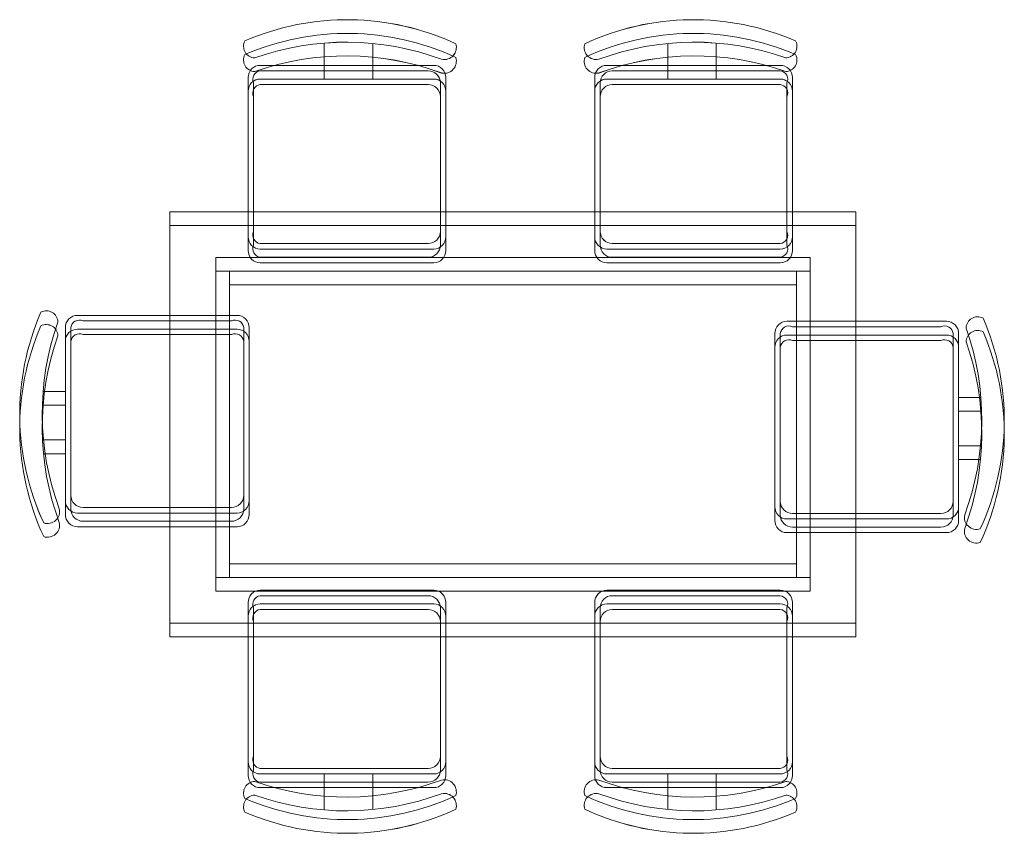
# Model space of a CAD drawing. Units: inches. Extents: x 963 to 2075, y 289 to 2657.
# Tile 90 of 98: x 1729 to 1781, y 2240 to 2282. Entities that reach past the tile are written whole.
import ezdxf

# ---------------------------------------------------------------- set-up
doc = ezdxf.new("R2010")
doc.units = ezdxf.units.IN
doc.layers.add('A-FURN', color=8, linetype='Continuous', lineweight=18)

msp = doc.modelspace()

# ---------------------------------------------------------------- linework, layer by layer
at = {"layer": 'A-FURN'}
for points in [[(1741.759, 2280.462, -0.175809), (1751.513, 2280.388, 0.578392), (1752.252, 2281.201, 0.214524), (1741.241, 2281.348, 0.552014), (1741.759, 2280.462, -0.065079)], [(1741.759, 2280.461, -0.175809), (1751.513, 2280.388, 0.578392), (1752.252, 2281.2, 0.214524), (1741.241, 2281.348, 0.552014), (1741.759, 2280.461, -0.065079)], [(1759.724, 2280.388, -0.578392), (1758.985, 2281.201, -0.214524), (1769.995, 2281.348, -0.552014), (1769.478, 2280.462, 0.175809), (1759.724, 2280.388)], [(1759.724, 2280.388, -0.578392), (1758.985, 2281.2, -0.214524), (1769.995, 2281.348, -0.552014), (1769.478, 2280.461, 0.175809), (1759.724, 2280.388)], [(1741.759, 2279.746, -0.175809), (1751.513, 2279.672, 0.578392), (1752.252, 2280.484, 0.214524), (1741.241, 2280.632, 0.552014), (1741.759, 2279.746, -0.065079)], [(1741.759, 2279.745, -0.175809), (1751.513, 2279.671, 0.578392), (1752.252, 2280.484, 0.214524), (1741.241, 2280.632, 0.552014), (1741.759, 2279.745, -0.065079)], [(1759.724, 2279.672, -0.578392), (1758.985, 2280.484, -0.214524), (1769.995, 2280.632, -0.552014), (1769.478, 2279.746, 0.175809), (1759.724, 2279.672)], [(1759.724, 2279.671, -0.578392), (1758.985, 2280.484, -0.214524), (1769.995, 2280.632, -0.552014), (1769.478, 2279.745, 0.175809), (1759.724, 2279.671)], [(1747.918, 2280.07), (1747.918, 2281.216, -0.064759)], [(1747.918, 2280.07), (1747.918, 2281.215, -0.064759)], [(1763.319, 2280.07), (1763.319, 2281.216, 0.064759)], [(1763.319, 2280.07), (1763.319, 2281.215, 0.064759)], [(1747.918, 2279.354), (1747.918, 2280.499, -0.064759)], [(1747.918, 2279.354), (1747.918, 2280.499, -0.064759)], [(1763.319, 2279.354), (1763.319, 2280.499, 0.064759)], [(1763.319, 2279.354), (1763.319, 2280.499, 0.064759)], [(1751.099, 2280.07), (1742.044, 2280.07, 0.414214), (1741.41, 2279.437), (1741.41, 2271.111, 0.414214), (1742.044, 2270.477), (1751.099, 2270.477, 0.414214), (1751.732, 2271.111), (1751.732, 2279.437, 0.414214), (1751.099, 2280.07)], [(1751.099, 2280.07), (1742.044, 2280.07, 0.414214), (1741.41, 2279.437), (1741.41, 2271.11, 0.414214), (1742.044, 2270.477), (1751.099, 2270.477, 0.414214), (1751.732, 2271.11), (1751.732, 2279.437, 0.414214), (1751.099, 2280.07)], [(1769.193, 2280.07, -0.414214), (1769.827, 2279.437), (1769.827, 2271.111, -0.414214), (1769.193, 2270.477), (1760.138, 2270.477, -0.414214), (1759.504, 2271.111), (1759.504, 2279.437, -0.414214), (1760.138, 2280.07), (1769.193, 2280.07)], [(1769.193, 2280.07, -0.414214), (1769.827, 2279.437), (1769.827, 2271.11, -0.414214), (1769.193, 2270.477), (1760.138, 2270.477, -0.414214), (1759.504, 2271.11), (1759.504, 2279.437, -0.414214), (1760.138, 2280.07), (1769.193, 2280.07)], [(1751.099, 2279.354), (1742.044, 2279.354, 0.414214), (1741.41, 2278.721), (1741.41, 2270.395, 0.414214), (1742.044, 2269.761), (1751.099, 2269.761, 0.414214), (1751.732, 2270.395), (1751.732, 2278.721, 0.414214), (1751.099, 2279.354)], [(1751.099, 2279.354), (1742.044, 2279.354, 0.414214), (1741.41, 2278.72), (1741.41, 2270.394, 0.414214), (1742.044, 2269.761), (1751.099, 2269.761, 0.414214), (1751.732, 2270.394), (1751.732, 2278.72, 0.414214), (1751.099, 2279.354)], [(1769.193, 2279.354, -0.414214), (1769.827, 2278.721), (1769.827, 2270.395, -0.414214), (1769.193, 2269.761), (1760.138, 2269.761, -0.414214), (1759.504, 2270.395), (1759.504, 2278.721, -0.414214), (1760.138, 2279.354), (1769.193, 2279.354)], [(1769.193, 2279.354, -0.414214), (1769.827, 2278.72), (1769.827, 2270.394, -0.414214), (1769.193, 2269.761), (1760.138, 2269.761, -0.414214), (1759.504, 2270.394), (1759.504, 2278.72, -0.414214), (1760.138, 2279.354), (1769.193, 2279.354)], [(1731.554, 2256.908, -0.578392), (1730.742, 2256.169, -0.214524), (1730.594, 2267.179, -0.552014), (1731.48, 2266.662, 0.175809), (1731.554, 2256.908)], [(1731.554, 2256.907, -0.578392), (1730.742, 2256.168, -0.214524), (1730.594, 2267.178, -0.552014), (1731.48, 2266.661, 0.175809), (1731.554, 2256.907)], [(1731.872, 2266.377, -0.414214), (1732.505, 2267.01), (1740.831, 2267.01, -0.414214), (1741.465, 2266.377), (1741.465, 2257.321, -0.414214), (1740.831, 2256.688), (1732.505, 2256.688, -0.414214), (1731.872, 2257.321), (1731.872, 2266.377)], [(1731.872, 2266.376, -0.414214), (1732.505, 2267.01), (1740.831, 2267.01, -0.414214), (1741.465, 2266.376), (1741.465, 2257.321, -0.414214), (1740.831, 2256.688), (1732.505, 2256.688, -0.414214), (1731.872, 2257.321), (1731.872, 2266.376)], [(1778.893, 2266.351, -0.175809), (1778.82, 2256.598, 0.578392), (1779.632, 2255.859, 0.214524), (1779.78, 2266.869, 0.552014), (1778.893, 2266.351, -0.065079)], [(1778.893, 2266.351, -0.175809), (1778.82, 2256.597, 0.578392), (1779.632, 2255.858, 0.214524), (1779.78, 2266.868, 0.552014), (1778.893, 2266.351, -0.065079)], [(1731.554, 2256.191, -0.578392), (1730.742, 2255.452, -0.214524), (1730.594, 2266.463, -0.552014), (1731.48, 2265.945, 0.175809), (1731.554, 2256.191)], [(1731.554, 2256.191, -0.578392), (1730.742, 2255.452, -0.214524), (1730.594, 2266.462, -0.552014), (1731.48, 2265.945, 0.175809), (1731.554, 2256.191)], [(1778.502, 2266.067, 0.414214), (1777.868, 2266.7), (1769.542, 2266.7, 0.414214), (1768.909, 2266.067), (1768.909, 2257.011, 0.414214), (1769.542, 2256.378), (1777.868, 2256.378, 0.414214), (1778.502, 2257.011), (1778.502, 2266.067)], [(1778.502, 2266.066, 0.414214), (1777.868, 2266.7), (1769.542, 2266.7, 0.414214), (1768.909, 2266.066), (1768.909, 2257.011, 0.414214), (1769.542, 2256.377), (1777.868, 2256.377, 0.414214), (1778.502, 2257.011), (1778.502, 2266.066)], [(1731.872, 2265.66, -0.414214), (1732.505, 2266.294), (1740.831, 2266.294, -0.414214), (1741.465, 2265.66), (1741.465, 2256.605, -0.414214), (1740.831, 2255.972), (1732.505, 2255.972, -0.414214), (1731.872, 2256.605), (1731.872, 2265.66)], [(1731.872, 2265.66, -0.414214), (1732.505, 2266.294), (1740.831, 2266.294, -0.414214), (1741.465, 2265.66), (1741.465, 2256.605, -0.414214), (1740.831, 2255.971), (1732.505, 2255.971, -0.414214), (1731.872, 2256.605), (1731.872, 2265.66)], [(1778.502, 2265.35, 0.414214), (1777.868, 2265.984), (1769.542, 2265.984, 0.414214), (1768.909, 2265.35), (1768.909, 2256.295, 0.414214), (1769.542, 2255.662), (1777.868, 2255.662, 0.414214), (1778.502, 2256.295), (1778.502, 2265.35)], [(1778.502, 2265.35, 0.414214), (1777.868, 2265.983), (1769.542, 2265.983, 0.414214), (1768.909, 2265.35), (1768.909, 2256.295, 0.414214), (1769.542, 2255.661), (1777.868, 2255.661, 0.414214), (1778.502, 2256.295), (1778.502, 2265.35)], [(1778.893, 2265.635, -0.175809), (1778.82, 2255.881, 0.578392), (1779.632, 2255.142, 0.214524), (1779.78, 2266.152, 0.552014), (1778.893, 2265.635, -0.065079)], [(1778.893, 2265.635, -0.175809), (1778.82, 2255.881, 0.578392), (1779.632, 2255.142, 0.214524), (1779.78, 2266.152, 0.552014), (1778.893, 2265.635, -0.065079)], [(1731.872, 2260.502), (1730.727, 2260.502, 0.064759)], [(1731.872, 2260.502), (1730.727, 2260.502, 0.064759)], [(1778.502, 2260.192), (1779.647, 2260.192, -0.064759)], [(1778.502, 2260.192), (1779.647, 2260.192, -0.064759)], [(1731.872, 2259.786), (1730.727, 2259.786, 0.064759)], [(1731.872, 2259.786), (1730.727, 2259.786, 0.064759)], [(1778.502, 2259.476), (1779.647, 2259.476, -0.064759)], [(1778.502, 2259.475), (1779.647, 2259.475, -0.064759)], [(1751.099, 2243.059), (1742.044, 2243.059, -0.414214), (1741.41, 2243.692), (1741.41, 2252.019, -0.414214), (1742.044, 2252.652), (1751.099, 2252.652, -0.414214), (1751.732, 2252.019), (1751.732, 2243.692, -0.414214), (1751.099, 2243.059)], [(1751.099, 2243.059), (1742.044, 2243.059, -0.414214), (1741.41, 2243.692), (1741.41, 2252.018, -0.414214), (1742.044, 2252.652), (1751.099, 2252.652, -0.414214), (1751.732, 2252.018), (1751.732, 2243.692, -0.414214), (1751.099, 2243.059)], [(1769.193, 2243.059, 0.414214), (1769.827, 2243.692), (1769.827, 2252.019, 0.414214), (1769.193, 2252.652), (1760.138, 2252.652, 0.414214), (1759.504, 2252.019), (1759.504, 2243.692, 0.414214), (1760.138, 2243.059), (1769.193, 2243.059)], [(1769.193, 2243.059, 0.414214), (1769.827, 2243.692), (1769.827, 2252.018, 0.414214), (1769.193, 2252.652), (1760.138, 2252.652, 0.414214), (1759.504, 2252.018), (1759.504, 2243.692, 0.414214), (1760.138, 2243.059), (1769.193, 2243.059)], [(1751.099, 2242.343), (1742.044, 2242.343, -0.414214), (1741.41, 2242.976), (1741.41, 2251.302, -0.414214), (1742.044, 2251.936), (1751.099, 2251.936, -0.414214), (1751.732, 2251.302), (1751.732, 2242.976, -0.414214), (1751.099, 2242.343)], [(1751.099, 2242.342), (1742.044, 2242.342, -0.414214), (1741.41, 2242.976), (1741.41, 2251.302, -0.414214), (1742.044, 2251.935), (1751.099, 2251.935, -0.414214), (1751.732, 2251.302), (1751.732, 2242.976, -0.414214), (1751.099, 2242.342)], [(1769.193, 2242.343, 0.414214), (1769.827, 2242.976), (1769.827, 2251.302, 0.414214), (1769.193, 2251.936), (1760.138, 2251.936, 0.414214), (1759.504, 2251.302), (1759.504, 2242.976, 0.414214), (1760.138, 2242.343), (1769.193, 2242.343)], [(1769.193, 2242.342, 0.414214), (1769.827, 2242.976), (1769.827, 2251.302, 0.414214), (1769.193, 2251.935), (1760.138, 2251.935, 0.414214), (1759.504, 2251.302), (1759.504, 2242.976, 0.414214), (1760.138, 2242.342), (1769.193, 2242.342)], [(1751.513, 2242.741, -0.578392), (1752.252, 2241.929, -0.214524), (1741.241, 2241.781, -0.552014), (1741.759, 2242.667, 0.175809), (1751.513, 2242.741)], [(1751.513, 2242.741, -0.578392), (1752.252, 2241.928, -0.214524), (1741.241, 2241.781, -0.552014), (1741.759, 2242.667, 0.175809), (1751.513, 2242.741)], [(1747.918, 2243.059), (1747.918, 2241.914, 0.064759)], [(1747.918, 2243.059), (1747.918, 2241.913, 0.064759)], [(1769.478, 2242.667, -0.175809), (1759.724, 2242.741, 0.578392), (1758.985, 2241.929, 0.214524), (1769.995, 2241.781, 0.552014), (1769.478, 2242.667, -0.065079)], [(1769.478, 2242.667, -0.175809), (1759.724, 2242.741, 0.578392), (1758.985, 2241.928, 0.214524), (1769.995, 2241.781, 0.552014), (1769.478, 2242.667, -0.065079)], [(1763.319, 2243.059), (1763.319, 2241.914, -0.064759)], [(1763.319, 2243.059), (1763.319, 2241.913, -0.064759)], [(1747.918, 2242.343), (1747.918, 2241.197, 0.064759)], [(1747.918, 2242.342), (1747.918, 2241.197, 0.064759)], [(1763.319, 2242.343), (1763.319, 2241.197, -0.064759)], [(1763.319, 2242.342), (1763.319, 2241.197, -0.064759)], [(1751.513, 2242.025, -0.578392), (1752.252, 2241.213, -0.214524), (1741.241, 2241.065, -0.552014), (1741.759, 2241.951, 0.175809), (1751.513, 2242.025)], [(1751.513, 2242.025, -0.578392), (1752.252, 2241.212, -0.214524), (1741.241, 2241.064, -0.552014), (1741.759, 2241.951, 0.175809), (1751.513, 2242.025)], [(1769.478, 2241.951, -0.175809), (1759.724, 2242.025, 0.578392), (1758.985, 2241.213, 0.214524), (1769.995, 2241.065, 0.552014), (1769.478, 2241.951, -0.065079)], [(1769.478, 2241.951, -0.175809), (1759.724, 2242.025, 0.578392), (1758.985, 2241.212, 0.214524), (1769.995, 2241.064, 0.552014), (1769.478, 2241.951, -0.065079)]]:
    msp.add_lwpolyline(points, format="xyb", dxfattribs=at)
for points in [[(1745.383, 2281.236), (1745.383, 2280.07)], [(1745.383, 2281.236), (1745.383, 2280.07)], [(1765.853, 2281.236), (1765.853, 2280.07)], [(1765.853, 2281.236), (1765.853, 2280.07)], [(1745.383, 2280.52), (1745.383, 2279.354)], [(1745.383, 2280.52), (1745.383, 2279.354)], [(1765.853, 2280.52), (1765.853, 2279.354)], [(1765.853, 2280.52), (1765.853, 2279.354)], [(1730.706, 2263.037), (1731.872, 2263.037)], [(1730.706, 2263.036), (1731.872, 2263.036)], [(1730.706, 2262.321), (1731.872, 2262.321)], [(1730.706, 2262.32), (1731.872, 2262.32)], [(1779.668, 2262.727), (1778.502, 2262.727)], [(1779.668, 2262.726), (1778.502, 2262.726)], [(1779.668, 2262.01), (1778.502, 2262.01)], [(1779.668, 2262.01), (1778.502, 2262.01)], [(1745.383, 2241.893), (1745.383, 2243.059)], [(1745.383, 2241.893), (1745.383, 2243.059)], [(1765.853, 2241.893), (1765.853, 2243.059)], [(1765.853, 2241.893), (1765.853, 2243.059)], [(1745.383, 2241.177), (1745.383, 2242.343)], [(1745.383, 2241.176), (1745.383, 2242.342)], [(1765.853, 2241.177), (1765.853, 2242.343)], [(1765.853, 2241.176), (1765.853, 2242.342)]]:
    msp.add_lwpolyline(points, dxfattribs=at)
for points in [[(1742.047, 2279.785), (1750.813, 2279.785, -0.414214), (1751.447, 2279.151), (1751.447, 2271.396, -0.414214), (1750.813, 2270.763), (1742.047, 2270.763, -0.512069), (1741.695, 2271.396), (1741.695, 2279.151, -0.512069)], [(1742.047, 2279.785), (1750.813, 2279.785, -0.414214), (1751.447, 2279.151), (1751.447, 2271.396, -0.414214), (1750.813, 2270.762), (1742.047, 2270.762, -0.512069), (1741.696, 2271.396), (1741.696, 2279.151, -0.512069)], [(1769.189, 2279.785), (1760.423, 2279.785, 0.414214), (1759.79, 2279.151), (1759.79, 2271.396, 0.414214), (1760.423, 2270.763), (1769.189, 2270.763, 0.512069), (1769.541, 2271.396), (1769.541, 2279.151, 0.512069)], [(1769.189, 2279.785), (1760.423, 2279.785, 0.414214), (1759.79, 2279.151), (1759.79, 2271.396, 0.414214), (1760.423, 2270.762), (1769.189, 2270.762, 0.512069), (1769.541, 2271.396), (1769.541, 2279.151, 0.512069)], [(1742.047, 2279.069), (1750.813, 2279.069, -0.414214), (1751.447, 2278.435), (1751.447, 2270.68, -0.414214), (1750.813, 2270.046), (1742.047, 2270.046, -0.512069), (1741.695, 2270.68), (1741.695, 2278.435, -0.512069)], [(1742.047, 2279.068), (1750.813, 2279.068, -0.414214), (1751.447, 2278.435), (1751.447, 2270.68, -0.414214), (1750.813, 2270.046), (1742.047, 2270.046, -0.512069), (1741.696, 2270.68), (1741.696, 2278.435, -0.512069)], [(1769.189, 2279.069), (1760.423, 2279.069, 0.414214), (1759.79, 2278.435), (1759.79, 2270.68, 0.414214), (1760.423, 2270.046), (1769.189, 2270.046, 0.512069), (1769.541, 2270.68), (1769.541, 2278.435, 0.512069)], [(1769.189, 2279.068), (1760.423, 2279.068, 0.414214), (1759.79, 2278.435), (1759.79, 2270.68, 0.414214), (1760.423, 2270.046), (1769.189, 2270.046, 0.512069), (1769.541, 2270.68), (1769.541, 2278.435, 0.512069)], [(1732.157, 2266.373), (1732.157, 2257.607, 0.414214), (1732.791, 2256.973), (1740.546, 2256.973, 0.414214), (1741.18, 2257.607), (1741.18, 2266.373, 0.512069), (1740.546, 2266.725), (1732.791, 2266.725, 0.512069)], [(1732.157, 2266.372), (1732.157, 2257.606, 0.414214), (1732.791, 2256.973), (1740.546, 2256.973, 0.414214), (1741.18, 2257.606), (1741.18, 2266.372, 0.512069), (1740.546, 2266.724), (1732.791, 2266.724, 0.512069)], [(1778.217, 2266.063), (1778.217, 2257.297, -0.414214), (1777.583, 2256.663), (1769.828, 2256.663, -0.414214), (1769.194, 2257.297), (1769.194, 2266.063, -0.512069), (1769.828, 2266.415), (1777.583, 2266.415, -0.512069)], [(1778.217, 2266.062), (1778.217, 2257.296, -0.414214), (1777.583, 2256.663), (1769.828, 2256.663, -0.414214), (1769.194, 2257.296), (1769.194, 2266.062, -0.512069), (1769.828, 2266.414), (1777.583, 2266.414, -0.512069)], [(1732.157, 2265.657), (1732.157, 2256.891, 0.414214), (1732.791, 2256.257), (1740.546, 2256.257, 0.414214), (1741.18, 2256.891), (1741.18, 2265.657, 0.512069), (1740.546, 2266.009), (1732.791, 2266.009, 0.512069)], [(1732.157, 2265.656), (1732.157, 2256.89, 0.414214), (1732.791, 2256.257), (1740.546, 2256.257, 0.414214), (1741.18, 2256.89), (1741.18, 2265.656, 0.512069), (1740.546, 2266.008), (1732.791, 2266.008, 0.512069)], [(1778.217, 2265.346), (1778.217, 2256.581, -0.414214), (1777.583, 2255.947), (1769.828, 2255.947, -0.414214), (1769.194, 2256.581), (1769.194, 2265.346, -0.512069), (1769.828, 2265.698), (1777.583, 2265.698, -0.512069)], [(1778.217, 2265.346), (1778.217, 2256.58, -0.414214), (1777.583, 2255.947), (1769.828, 2255.947, -0.414214), (1769.194, 2256.58), (1769.194, 2265.346, -0.512069), (1769.828, 2265.698), (1777.583, 2265.698, -0.512069)], [(1742.047, 2243.344), (1750.813, 2243.344, 0.414214), (1751.447, 2243.978), (1751.447, 2251.733, 0.414214), (1750.813, 2252.367), (1742.047, 2252.367, 0.512069), (1741.695, 2251.733), (1741.695, 2243.978, 0.512069)], [(1742.047, 2243.344), (1750.813, 2243.344, 0.414214), (1751.447, 2243.977), (1751.447, 2251.733, 0.414214), (1750.813, 2252.366), (1742.047, 2252.366, 0.512069), (1741.696, 2251.733), (1741.696, 2243.977, 0.512069)], [(1769.189, 2243.344), (1760.423, 2243.344, -0.414214), (1759.79, 2243.978), (1759.79, 2251.733, -0.414214), (1760.423, 2252.367), (1769.189, 2252.367, -0.512069), (1769.541, 2251.733), (1769.541, 2243.978, -0.512069)], [(1769.189, 2243.344), (1760.423, 2243.344, -0.414214), (1759.79, 2243.977), (1759.79, 2251.733, -0.414214), (1760.423, 2252.366), (1769.189, 2252.366, -0.512069), (1769.541, 2251.733), (1769.541, 2243.977, -0.512069)], [(1742.047, 2242.628), (1750.813, 2242.628, 0.414214), (1751.447, 2243.262), (1751.447, 2251.017, 0.414214), (1750.813, 2251.65), (1742.047, 2251.65, 0.512069), (1741.695, 2251.017), (1741.695, 2243.262, 0.512069)], [(1742.047, 2242.628), (1750.813, 2242.628, 0.414214), (1751.447, 2243.261), (1751.447, 2251.017, 0.414214), (1750.813, 2251.65), (1742.047, 2251.65, 0.512069), (1741.696, 2251.017), (1741.696, 2243.261, 0.512069)], [(1769.189, 2242.628), (1760.423, 2242.628, -0.414214), (1759.79, 2243.262), (1759.79, 2251.017, -0.414214), (1760.423, 2251.65), (1769.189, 2251.65, -0.512069), (1769.541, 2251.017), (1769.541, 2243.262, -0.512069)], [(1769.189, 2242.628), (1760.423, 2242.628, -0.414214), (1759.79, 2243.261), (1759.79, 2251.017, -0.414214), (1760.423, 2251.65), (1769.189, 2251.65, -0.512069), (1769.541, 2251.017), (1769.541, 2243.261, -0.512069)]]:
    msp.add_lwpolyline(points, format="xyb", close=True, dxfattribs=at)
for points in [[(1737.329, 2272.423), (1773.14, 2272.423), (1773.14, 2250.936), (1737.329, 2250.936)], [(1737.329, 2272.423), (1773.14, 2272.423), (1773.14, 2250.936), (1737.329, 2250.936)], [(1737.329, 2271.707), (1773.14, 2271.707), (1773.14, 2250.22), (1737.329, 2250.22)], [(1737.329, 2271.706), (1773.14, 2271.706), (1773.14, 2250.22), (1737.329, 2250.22)], [(1739.717, 2270.036), (1770.753, 2270.036), (1770.753, 2253.324), (1739.717, 2253.324)], [(1739.717, 2270.035), (1770.753, 2270.035), (1770.753, 2253.323), (1739.717, 2253.323)], [(1739.717, 2269.319), (1770.753, 2269.319), (1770.753, 2252.608), (1739.717, 2252.608)], [(1739.717, 2269.319), (1770.753, 2269.319), (1770.753, 2252.607), (1739.717, 2252.607)], [(1740.433, 2269.319), (1770.037, 2269.319), (1770.037, 2254.04), (1740.433, 2254.04)], [(1740.433, 2269.319), (1770.037, 2269.319), (1770.037, 2254.04), (1740.433, 2254.04)], [(1740.433, 2268.603), (1770.037, 2268.603), (1770.037, 2253.324), (1740.433, 2253.324)], [(1740.433, 2268.603), (1770.037, 2268.603), (1770.037, 2253.323), (1740.433, 2253.323)]]:
    msp.add_lwpolyline(points, close=True, dxfattribs=at)

doc.saveas('drawing.dxf')
